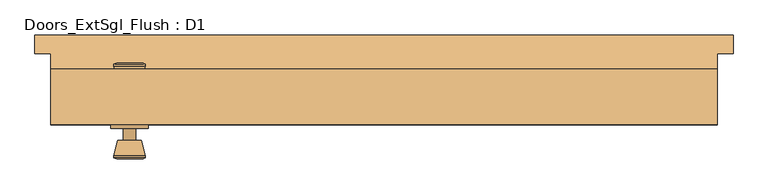
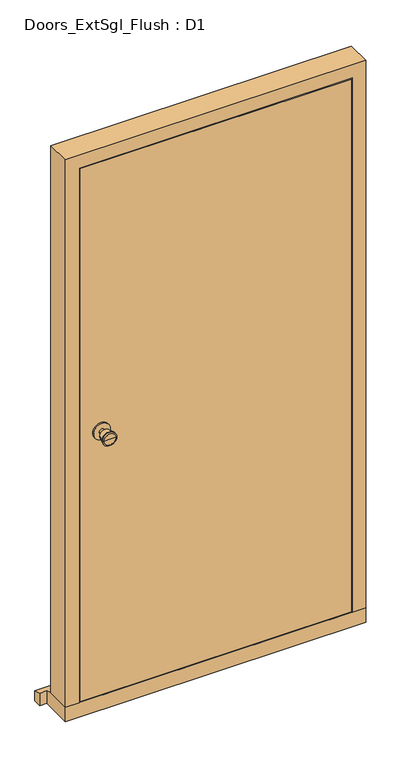
"""IFC4 building model written with IfcOpenShell, lengths in millimetres: door geometry, Doors_ExtSgl_Flush : D1."""

from ifc_helpers import new_model, si_unit, point, frame, frame_2d, origin, place, context, project, spatial, polyline, circle_curve, trimmed, segment, composite_curve, outline, extrude, faceted_brep, source, transform, mapped, element, save
from ifc_brep_helpers import plane_surface, cylinder_surface, revolved_surface, advanced_brep


def doors_extsgl_flush_d1_11f69a25(model_context):
    return source(origin(), model_context, "Body", "SolidModel", [
        advanced_brep(
        [(-406.9, -43.8, 1050.0), (-396.9, -43.8, 1050.0), (-416.9, -43.8, 1050.0), (-386.4241324, -92.8, 1050.0), (-406.9, -92.8, 1050.0), (-427.3758676, -92.8, 1050.0), (-381.9, -90.9721319, 1050.0), (-431.9, -90.9721319, 1050.0), (-381.9, -87.5084537, 1050.0), (-431.9, -87.5084537, 1050.0), (-388.263764, -62.8, 1050.0), (-425.536236, -62.8, 1050.0), (-396.9, -62.8, 1050.0), (-416.9, -62.8, 1050.0)],
        [
            (0, 1),
            (1, 2, circle_curve(frame((-406.9, -43.8, 1050.0), z_axis=(0.0, 1.0, 0.0), x_axis=(-1.0, 0.0, 0.0)), 10.0)),
            (2, 0),
            (2, 1, circle_curve(frame((-406.9, -43.8, 1050.0), z_axis=(0.0, 1.0, 0.0), x_axis=(-1.0, 0.0, 0.0)), 10.0)),
            (3, 4),
            (4, 5),
            (5, 3, circle_curve(frame((-406.9, -92.8, 1050.0), z_axis=(0.0, -1.0, 0.0), x_axis=(-1.0, 0.0, 0.0)), 20.4758676)),
            (3, 5, circle_curve(frame((-406.9, -92.8, 1050.0), z_axis=(0.0, -1.0, 0.0), x_axis=(-1.0, 0.0, 0.0)), 20.4758676)),
            (6, 3),
            (5, 7),
            (7, 6, circle_curve(frame((-406.9, -90.9721319, 1050.0), z_axis=(0.0, -1.0, 0.0), x_axis=(-1.0, 0.0, 0.0)), 25.0)),
            (6, 7, circle_curve(frame((-406.9, -90.9721319, 1050.0), z_axis=(0.0, -1.0, 0.0), x_axis=(-1.0, 0.0, 0.0)), 25.0)),
            (8, 6),
            (7, 9),
            (9, 8, circle_curve(frame((-406.9, -87.5084537, 1050.0), z_axis=(0.0, -1.0, 0.0), x_axis=(-1.0, 0.0, 0.0)), 25.0)),
            (8, 9, circle_curve(frame((-406.9, -87.5084537, 1050.0), z_axis=(0.0, -1.0, 0.0), x_axis=(-1.0, 0.0, 0.0)), 25.0)),
            (10, 8),
            (9, 11),
            (11, 10, circle_curve(frame((-406.9, -62.8, 1050.0), z_axis=(0.0, -1.0, 0.0), x_axis=(-1.0, 0.0, 0.0)), 18.636236)),
            (10, 11, circle_curve(frame((-406.9, -62.8, 1050.0), z_axis=(0.0, -1.0, 0.0), x_axis=(-1.0, 0.0, 0.0)), 18.636236)),
            (12, 10),
            (11, 13),
            (13, 12, circle_curve(frame((-406.9, -62.8, 1050.0), z_axis=(0.0, -1.0, 0.0), x_axis=(-1.0, 0.0, 0.0)), 10.0)),
            (12, 13, circle_curve(frame((-406.9, -62.8, 1050.0), z_axis=(0.0, -1.0, 0.0), x_axis=(-1.0, 0.0, 0.0)), 10.0)),
            (1, 12),
            (13, 2),
        ],
        [
            plane_surface(frame((-406.9, -43.8, 1050.0), z_axis=(0.0, 1.0, 0.0), x_axis=(-1.0, 0.0, 0.0))),
            plane_surface(frame((-406.9, -92.8, 1050.0), z_axis=(0.0, -1.0, 0.0), x_axis=(-1.0, 0.0, 0.0))),
            revolved_surface(polyline([(-427.3758676, -92.8, 1050.0), (-431.9, -90.9721319, 1050.0)]), (-406.9, -43.8, 1050.0), (0.0, 1.0, 0.0)),
            cylinder_surface(frame((-406.9, -43.8, 1050.0), z_axis=(0.0, 1.0, 0.0), x_axis=(-1.0, 0.0, 0.0)), 25.0),
            revolved_surface(polyline([(-431.9, -87.5084537, 1050.0), (-425.536236, -62.8, 1050.0)]), (-406.9, -43.8, 1050.0), (0.0, 1.0, 0.0)),
            plane_surface(frame((-406.9, -62.8, 1050.0), z_axis=(0.0, 1.0, 0.0), x_axis=(-1.0, 0.0, 0.0))),
            cylinder_surface(frame((-406.9, -43.8, 1050.0), z_axis=(0.0, 1.0, 0.0), x_axis=(-1.0, 0.0, 0.0)), 10.0),
        ],
        [
            (0, [[1, 2, 3]]),
            (0, [[-3, 4, -1]]),
            (1, [[5, 6, 7]]),
            (1, [[-6, -5, 8]]),
            (2, [[9, -7, 10, 11]]),
            (2, [[-10, -8, -9, 12]]),
            (3, [[13, -11, 14, 15]]),
            (3, [[-14, -12, -13, 16]]),
            (4, [[17, -15, 18, 19]]),
            (4, [[-18, -16, -17, 20]]),
            (5, [[21, -19, 22, 23]]),
            (5, [[-22, -20, -21, 24]]),
            (6, [[25, -23, 26, -2]]),
            (6, [[-26, -24, -25, -4]]),
        ],
    ),
        extrude(outline(composite_curve([segment(trimmed(circle_curve(frame_2d((1050.0, -406.9)), 30.0), [point((1050.0, -436.9))], [point((1050.0, -376.9))], False, "CARTESIAN"), True, "CONTINUOUS"), segment(trimmed(circle_curve(frame_2d((1050.0, -406.9)), 30.0), [point((1050.0, -376.9))], [point((1050.0, -436.9))], False, "CARTESIAN"), True, "CONTINUOUS")], self_intersect=False)), frame((0.0, -43.8, 0.0), z_axis=(0.0, 1.0, 0.0), x_axis=(0.0, 0.0, 1.0)), (0.0, 0.0, 1.0), 6.0),
        advanced_brep(
        [(-406.9, 12.2, 1050.0), (-416.9, 12.2, 1050.0), (-396.9, 12.2, 1050.0), (-386.4241324, 61.2, 1050.0), (-427.3758676, 61.2, 1050.0), (-406.9, 61.2, 1050.0), (-381.9, 59.3721319, 1050.0), (-431.9, 59.3721319, 1050.0), (-381.9, 55.9084537, 1050.0), (-431.9, 55.9084537, 1050.0), (-388.263764, 31.2, 1050.0), (-425.536236, 31.2, 1050.0), (-396.9, 31.2, 1050.0), (-416.9, 31.2, 1050.0)],
        [
            (0, 1),
            (1, 2, circle_curve(frame((-406.9, 12.2, 1050.0), z_axis=(0.0, -1.0, 0.0), x_axis=(-1.0, 0.0, 0.0)), 10.0)),
            (2, 0),
            (2, 1, circle_curve(frame((-406.9, 12.2, 1050.0), z_axis=(0.0, -1.0, 0.0), x_axis=(-1.0, 0.0, 0.0)), 10.0)),
            (3, 4, circle_curve(frame((-406.9, 61.2, 1050.0), z_axis=(0.0, 1.0, 0.0), x_axis=(-1.0, 0.0, 0.0)), 20.4758676)),
            (4, 5),
            (5, 3),
            (4, 3, circle_curve(frame((-406.9, 61.2, 1050.0), z_axis=(0.0, 1.0, 0.0), x_axis=(-1.0, 0.0, 0.0)), 20.4758676)),
            (6, 7, circle_curve(frame((-406.9, 59.3721319, 1050.0), z_axis=(0.0, 1.0, 0.0), x_axis=(-1.0, 0.0, 0.0)), 25.0)),
            (7, 4),
            (3, 6),
            (7, 6, circle_curve(frame((-406.9, 59.3721319, 1050.0), z_axis=(0.0, 1.0, 0.0), x_axis=(-1.0, 0.0, 0.0)), 25.0)),
            (8, 9, circle_curve(frame((-406.9, 55.9084537, 1050.0), z_axis=(0.0, 1.0, 0.0), x_axis=(-1.0, 0.0, 0.0)), 25.0)),
            (9, 7),
            (6, 8),
            (9, 8, circle_curve(frame((-406.9, 55.9084537, 1050.0), z_axis=(0.0, 1.0, 0.0), x_axis=(-1.0, 0.0, 0.0)), 25.0)),
            (10, 11, circle_curve(frame((-406.9, 31.2, 1050.0), z_axis=(0.0, 1.0, 0.0), x_axis=(-1.0, 0.0, 0.0)), 18.636236)),
            (11, 9),
            (8, 10),
            (11, 10, circle_curve(frame((-406.9, 31.2, 1050.0), z_axis=(0.0, 1.0, 0.0), x_axis=(-1.0, 0.0, 0.0)), 18.636236)),
            (12, 13, circle_curve(frame((-406.9, 31.2, 1050.0), z_axis=(0.0, 1.0, 0.0), x_axis=(-1.0, 0.0, 0.0)), 10.0)),
            (13, 11),
            (10, 12),
            (13, 12, circle_curve(frame((-406.9, 31.2, 1050.0), z_axis=(0.0, 1.0, 0.0), x_axis=(-1.0, 0.0, 0.0)), 10.0)),
            (1, 13),
            (12, 2),
        ],
        [
            plane_surface(frame((-406.9, 12.2, 1050.0), z_axis=(0.0, -1.0, 0.0), x_axis=(-1.0, 0.0, 0.0))),
            plane_surface(frame((-406.9, 61.2, 1050.0), z_axis=(0.0, 1.0, 0.0), x_axis=(-1.0, 0.0, 0.0))),
            revolved_surface(polyline([(-427.3758676, 61.2, 1050.0), (-431.9, 59.3721319, 1050.0)]), (-406.9, 12.2, 1050.0), (0.0, -1.0, 0.0)),
            cylinder_surface(frame((-406.9, 12.2, 1050.0), z_axis=(0.0, -1.0, 0.0), x_axis=(-1.0, 0.0, 0.0)), 25.0),
            revolved_surface(polyline([(-431.9, 55.9084537, 1050.0), (-425.536236, 31.2, 1050.0)]), (-406.9, 12.2, 1050.0), (0.0, -1.0, 0.0)),
            plane_surface(frame((-406.9, 31.2, 1050.0), z_axis=(0.0, -1.0, 0.0), x_axis=(-1.0, 0.0, 0.0))),
            cylinder_surface(frame((-406.9, 12.2, 1050.0), z_axis=(0.0, -1.0, 0.0), x_axis=(-1.0, 0.0, 0.0)), 10.0),
        ],
        [
            (0, [[1, 2, 3]]),
            (0, [[-3, 4, -1]]),
            (1, [[5, 6, 7]]),
            (1, [[8, -7, -6]]),
            (2, [[9, 10, -5, 11]]),
            (2, [[12, -11, -8, -10]]),
            (3, [[13, 14, -9, 15]]),
            (3, [[16, -15, -12, -14]]),
            (4, [[17, 18, -13, 19]]),
            (4, [[20, -19, -16, -18]]),
            (5, [[21, 22, -17, 23]]),
            (5, [[24, -23, -20, -22]]),
            (6, [[-2, 25, -21, 26]]),
            (6, [[-4, -26, -24, -25]]),
        ],
    ),
        extrude(outline(composite_curve([segment(trimmed(circle_curve(frame_2d((1050.0, -406.9)), 30.0), [point((1050.0, -436.9))], [point((1050.0, -376.9))], False, "CARTESIAN"), True, "CONTINUOUS"), segment(trimmed(circle_curve(frame_2d((1050.0, -406.9)), 30.0), [point((1050.0, -376.9))], [point((1050.0, -436.9))], False, "CARTESIAN"), True, "CONTINUOUS")], self_intersect=False)), frame((0.0, 6.2, 0.0), z_axis=(0.0, 1.0, 0.0), x_axis=(0.0, 0.0, 1.0)), (0.0, 0.0, 1.0), 6.0),
        faceted_brep([(462.9, 51.2, 54.5), (533.4, 51.2, 54.5), (533.4, -37.8, 54.5), (484.9, -37.8, 54.5), (484.9, 9.2, 54.5), (462.9, 9.2, 54.5), (462.9, 51.2, 2039.5), (-462.9, 51.2, 2039.5), (-462.9, 51.2, 54.5), (-533.4, 51.2, 54.5), (-533.4, 51.2, 2110.0), (533.4, 51.2, 2110.0), (533.4, -37.8, 2110.0), (-533.4, -37.8, 2110.0), (-533.4, -37.8, 54.5), (-484.9, -37.8, 54.5), (-484.9, -37.8, 2061.5), (484.9, -37.8, 2061.5), (484.9, 9.2, 2061.5), (-484.9, 9.2, 2061.5), (-484.9, 9.2, 54.5), (-462.9, 9.2, 54.5), (-462.9, 9.2, 2039.5), (462.9, 9.2, 2039.5)], [[[0, 1, 2, 3, 4, 5]], [[1, 0, 6, 7, 8, 9, 10, 11]], [[2, 1, 11, 12]], [[3, 2, 12, 13, 14, 15, 16, 17]], [[4, 3, 17, 18]], [[5, 4, 18, 19, 20, 21, 22, 23]], [[0, 5, 23, 6]], [[7, 22, 21, 8]], [[8, 21, 20, 15, 14, 9]], [[13, 10, 9, 14]], [[19, 16, 15, 20]], [[12, 11, 10, 13]], [[18, 17, 16, 19]], [[6, 23, 22, 7]]]),
        extrude(outline(polyline([(481.9, -37.8), (-482.8250294, -37.8), (-482.8250294, 6.2), (481.9, 6.2), (481.9, -37.8)])), frame((0.0, 0.0, 58.5), z_axis=(0.0, 0.0, 1.0), x_axis=(1.0, 0.0, 0.0)), (0.0, 0.0, 1.0), 2000.0),
        faceted_brep([(558.4, 106.2, 0.0), (558.4, 106.2, 38.5947221), (558.4, 76.2, 47.2703282), (558.4, 76.2, 0.0), (-558.4, 106.2, 38.5947221), (-558.4, 106.2, 0.0), (-558.4, 76.2, 0.0), (-558.4, 76.2, 47.2703282), (533.4, 76.2, 0.0), (533.4, -37.8, 0.0), (-533.4, -37.8, 0.0), (-533.4, 76.2, 0.0), (-533.4, 76.2, 47.2703282), (-533.4, 51.2, 54.5), (533.4, 51.2, 54.5), (533.4, 76.2, 47.2703282), (-533.4, -37.8, 54.5), (533.4, -37.8, 54.5)], [[[0, 1, 2, 3]], [[4, 5, 6, 7]], [[5, 0, 3, 8, 9, 10, 11, 6]], [[1, 0, 5, 4]], [[1, 4, 7, 12, 13, 14, 15, 2]], [[13, 16, 17, 14]], [[16, 10, 9, 17]], [[12, 11, 10, 16, 13]], [[11, 12, 7, 6]], [[8, 15, 14, 17, 9]], [[15, 8, 3, 2]]]),
    ])


if __name__ == "__main__":
    model = new_model("IFC4")
    model_context = context("Model", 3, world=origin())
    ifc_project = project(units=[si_unit("LENGTHUNIT", "METRE", prefix="MILLI")], contexts=[model_context])
    site = spatial("IfcSite", under=ifc_project)
    building = spatial("IfcBuilding", under=site)
    placement = place(None, origin())
    doors_extsgl_flush_d1_shape = doors_extsgl_flush_d1_11f69a25(model_context)
    element("IfcDoor", 1, ObjectType="Doors_ExtSgl_Flush : D1", at=placement, inside=building, context=model_context, shape_type="MappedRepresentation", body=[
        mapped(doors_extsgl_flush_d1_shape, transform((0.0, 0.0, 0.0), x_axis=(1.0, 0.0, 0.0), y_axis=(0.0, 1.0, 0.0), z_axis=(0.0, 0.0, 1.0))),
    ])
    save(model, "model.ifc")

# Revit data of these elements
# Type "Doors_ExtSgl_Flush : D1"
#   Type Mark = "49"
#   Type Comments = "External Single"
#   Operation = "SingleSwingRight"
#   Construction Type Id = "MDOOR"
#   Keynote = "L20"
#   Analytic Construction = "Metal"
#   Wrap Layers (Int) from Ext = 177.5 mm
#   Wrap Layers (Ext) from Ext = 102.5 mm
#   Thickness = 44 mm
#   Rough Width = 1066.8 mm
#   Rough Height = 2110 mm
#   O/A Frame Width = 64 mm
#   Heat Transfer Coefficient (U) = 3.7021 W/(m²·K)
#   Handle Z Distance = 1050 mm
#   FrameWidth = 42 mm
#   FrameOffset - External = 25 mm
#   FrameDepth = 89 mm
#   Door Panel Width = 963.8 mm
#   Door Panel Thickness = 44 mm
#   Door Panel Height = 2000 mm
#   Cill Thickness = 54.5 mm
#   Cill Projection = 30 mm
#   Handle X Distance = 75 mm
#   Height = 2110 mm
#   Structural Tolerance = 6.5 mm
#   Tolerance = 3 mm
#   Undercut = 4 mm
#   Width = 1066.8 mm
#   Cill Extension = 25 mm
#   Cavity Closer Width = 50 mm
#   Cavity Closer Offset from Ext = 102.5 mm
#   Cavity Closer Depth = 85 mm
#   Vis - Ironmongery = yes
#   Vis - Cavity Closers = yes
#   Define Thermal Properties by = 1
#   Function = 1
#   Material Door = Door - Panel
#   Material Frame = Door - Frame/Mullion
#   Material Ironmongery = Door - Handle
#   Visual Light Transmittance = 0
#   Solar Heat Gain Coefficient = 0
#   Wall Closure = (empty or 0)
# Element 1 (IfcDoor, "Doors_ExtSgl_Flush : D1")
#   Materials on its faces: "Door - Handle", "Door - Frame/Mullion", "Door - Panel"
# Materials
#   "Door - Panel": class "Wood", colour RGB 210 159 95, transparency 0, Keynote = "L20", Cost = 0
#   "Door - Frame/Mullion": class "Wood", colour RGB 212 179 113, transparency 0, Keynote = "L20", Cost = 0
#   "Door - Handle": colour RGB 0 0 0, transparency 0, Keynote = "P21", Cost = 0
